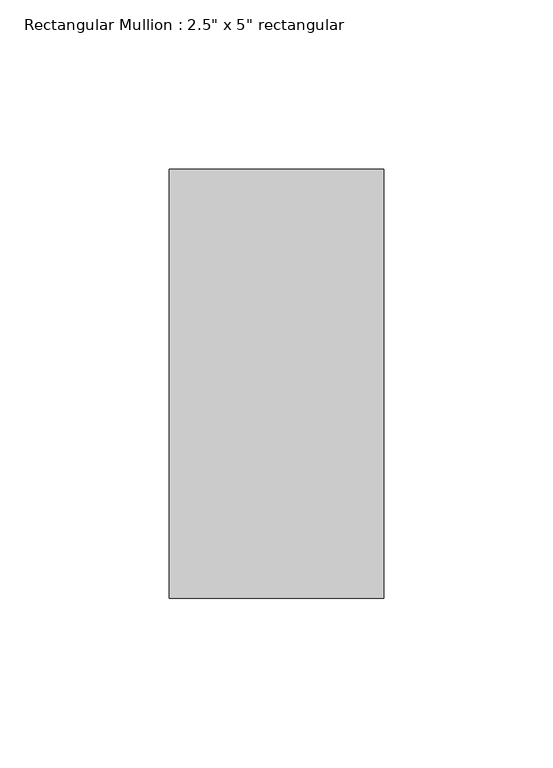
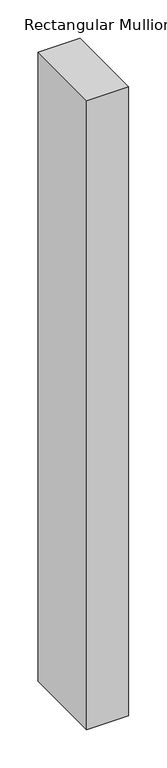
"""IFC4 building model written with IfcOpenShell, lengths in millimetres: member geometry."""

from ifc_helpers import new_model, si_unit, frame, origin, place, context, project, spatial, polyline, outline, extrude, source, transform, mapped, element, save


def member_cfcad22e(model_context):
    return source(origin(), model_context, "Body", "SweptSolid", [
        extrude(outline(polyline([(0.0, 63.5), (0.0, -63.5), (-63.5, -63.5), (-63.5, 63.5), (0.0, 63.5)])), frame((0.0, 0.0, -1003.3), z_axis=(0.0, 0.0, 1.0), x_axis=(1.0, 0.0, 0.0)), (0.0, 0.0, 1.0), 1003.3),
    ])


if __name__ == "__main__":
    model = new_model("IFC4")
    model_context = context("Model", 3, world=origin())
    ifc_project = project(units=[si_unit("LENGTHUNIT", "METRE", prefix="MILLI")], contexts=[model_context])
    site = spatial("IfcSite", under=ifc_project)
    building = spatial("IfcBuilding", under=site)
    placement = place(None, origin())
    member_shape = member_cfcad22e(model_context)
    element("IfcMember", 1, ObjectType="Rectangular Mullion : 2.5\" x 5\" rectangular", at=placement, inside=building, context=model_context, shape_type="MappedRepresentation", body=[
        mapped(member_shape, transform((0.0, 0.0, 0.0), x_axis=(1.0, 0.0, 0.0), y_axis=(0.0, 1.0, 0.0), z_axis=(0.0, 0.0, 1.0))),
    ])
    save(model, "model.ifc")

# Revit data of these elements
# Type "Rectangular Mullion : 2.5\" x 5\" rectangular"
#   built-in parameter 1007304 = 0.416667 (stored number, unit not read)
#   built-in parameter 1007301 = 0.104167 (stored number, unit not read)
#   built-in parameter 1007300 = 0.104167 (stored number, unit not read)
# Element 1 (IfcMember, "Rectangular Mullion : 2.5\" x 5\" rectangular")
#   Materials on its faces: "Iron, Ductile"
# Materials
#   "Iron, Ductile": class "Metal", colour RGB 0 0 0, transparency 0, Description = "Ductile cast iron", Cost = 0
